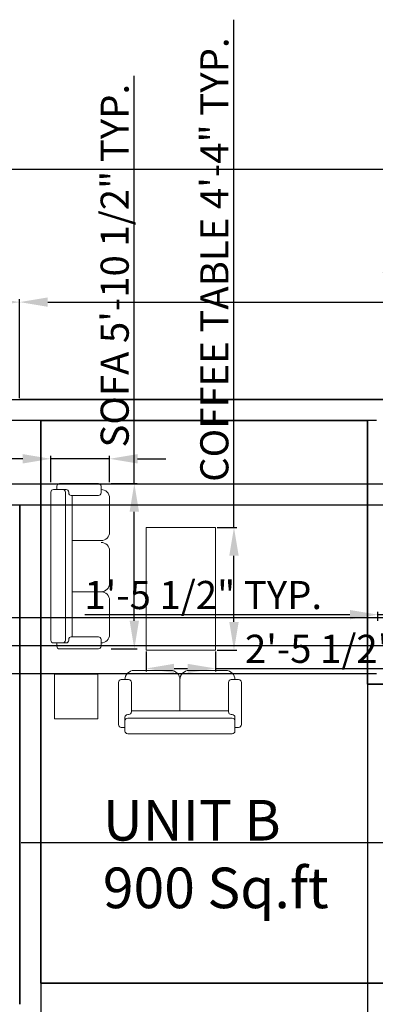
# Model space of a CAD drawing. Units: inches. Extents: x 2174 to 3353, y 1481 to 2316.
# Tile 7 of 8: x 2759 to 2911, y 1896 to 2316. Entities that reach past the tile are written whole.
import ezdxf

# ---------------------------------------------------------------- set-up
doc = ezdxf.new("R2010")
doc.units = ezdxf.units.IN
for name, color, linetype, lineweight in [('A-ANNO-DIMS', 2, 'Continuous', 18), ('A-AREA-IDEN', 7, 'Continuous', 25), ('A-FURN', 8, 'Continuous', 13), ('A-WALL', 7, 'Continuous', 35)]:
    doc.layers.add(name, color=color, linetype=linetype, lineweight=lineweight)
doc.styles.get("Standard").update_dxf_attribs({"font": 'arial.ttf'})
doc.dimstyles.new('ISO-25', dxfattribs={"dimtxt": 12, "dimasz": 12, "dimexe": 1.25, "dimexo": 0.625, "dimtad": 1, "dimlunit": 3, "dimtxsty": 'Standard', "dimcen": 2.5, "dimadec": 0, "dimazin": 0, "dimtfac": 1, "dimtmove": 0, "dimatfit": 3, "dimfxl": 1, "dimarcsym": 0})

# ---------------------------------------------------------------- blocks, each defined once
blk = doc.blocks.new('A$C115861F8')
for p, q in [((0, 0.572), (0, 0.126)), ((0.068, 0.601), (0.029, 0.601)), ((0.068, 0.64), (0.068, 0.601)), ((0.068, 0.533), (0.068, 0.601)), ((1.785, 0.669), (0.097, 0.669)), ((1.814, 0.64), (1.814, 0.601)), ((1.814, 0.601), (1.852, 0.601)), ((1.814, 0.533), (1.814, 0.601)), ((1.882, 0.572), (1.882, 0.126)), ((0.068, 0.495), (0.068, 0.543)), ((1.785, 0.504), (0.097, 0.504)), ((0.107, 0.466), (0.097, 0.466)), ((1.775, 0.466), (1.785, 0.466)), ((1.814, 0.495), (1.814, 0.543)), ((0.136, 0.126), (0.136, 0.436)), ((1.746, 0.427), (0.136, 0.427)), ((0.65, 0.097), (0.65, 0.427)), ((1.232, 0.097), (1.232, 0.427)), ((1.746, 0.126), (1.746, 0.436)), ((0.029, 0.097), (0.107, 0.097)), ((0.165, 0), (0.553, 0)), ((1.135, 0), (0.747, 0)), ((1.329, 0), (1.717, 0)), ((1.852, 0.097), (1.775, 0.097))]:
    blk.add_line(p, q)
for centre, radius, start, end in [((0.029, 0.572), 0.0291, 90, 180), ((0.097, 0.64), 0.0291, 90, 180), ((1.785, 0.64), 0.0291, 0, 90), ((1.852, 0.572), 0.0291, 0, 90), ((0.097, 0.533), 0.0291, 180, 270), ((0.097, 0.495), 0.0291, 180, 270), ((0.107, 0.436), 0.0291, 0, 90), ((1.775, 0.436), 0.0291, 90, 180), ((1.785, 0.533), 0.0291, 270, 0), ((1.785, 0.495), 0.0291, 270, 0), ((0.029, 0.126), 0.0291, 180, 270), ((0.107, 0.126), 0.0291, 270, 0), ((1.775, 0.126), 0.0291, 180, 270), ((1.852, 0.126), 0.0291, 270, 0), ((0.165, 0.097), 0.097, 180, 270), ((0.553, 0.097), 0.097, 270, 0), ((0.747, 0.097), 0.097, 180, 270), ((1.115, 0.097), 0.097, 270, 0), ((1.329, 0.097), 0.097, 180, 270), ((1.717, 0.097), 0.097, 270, 0)]:
    blk.add_arc(centre, radius, start, end)
blk = doc.blocks.new('A$C02A636C4')
for p, q in [((0.068, 0.64), (0.068, 0.601)), ((1.203, 0.669), (0.097, 0.669)), ((1.232, 0.64), (1.232, 0.601)), ((0, 0.572), (0, 0.126)), ((0.068, 0.601), (0.029, 0.601)), ((0.068, 0.533), (0.068, 0.601)), ((0.068, 0.495), (0.068, 0.543)), ((1.232, 0.601), (1.271, 0.601)), ((1.232, 0.533), (1.232, 0.601)), ((1.232, 0.495), (1.232, 0.543)), ((1.3, 0.572), (1.3, 0.126)), ((1.203, 0.504), (0.097, 0.504)), ((0.107, 0.466), (0.097, 0.466)), ((0.136, 0.126), (0.136, 0.436)), ((1.164, 0.427), (0.136, 0.427)), ((0.65, 0.097), (0.65, 0.427)), ((1.164, 0.126), (1.164, 0.436)), ((1.193, 0.466), (1.203, 0.466)), ((0.029, 0.097), (0.107, 0.097)), ((0.165, 0), (0.553, 0)), ((0.747, 0), (1.135, 0)), ((1.271, 0.097), (1.193, 0.097))]:
    blk.add_line(p, q)
for centre, radius, start, end in [((0.097, 0.64), 0.0291, 90, 180), ((1.203, 0.64), 0.0291, 0, 90), ((0.029, 0.572), 0.0291, 90, 180), ((0.097, 0.533), 0.0291, 180, 270), ((1.203, 0.533), 0.0291, 270, 0), ((1.271, 0.572), 0.0291, 0, 90), ((0.097, 0.495), 0.0291, 180, 270), ((0.107, 0.436), 0.0291, 0, 90), ((1.193, 0.436), 0.0291, 90, 180), ((1.203, 0.495), 0.0291, 270, 0), ((0.029, 0.126), 0.0291, 180, 270), ((0.107, 0.126), 0.0291, 270, 0), ((1.193, 0.126), 0.0291, 180, 270), ((1.271, 0.126), 0.0291, 270, 0), ((0.165, 0.097), 0.097, 180, 270), ((0.553, 0.097), 0.097, 270, 0), ((0.747, 0.097), 0.097, 180, 270), ((1.135, 0.097), 0.097, 270, 0)]:
    blk.add_arc(centre, radius, start, end)
blk = doc.blocks.new('*D7')
at = {"layer": 'A-ANNO-DIMS', "color": 0, "lineweight": -2, "transparency": 16777216}
for p, q in [((2285.44, 2154.23), (2285.44, 2253.16)), ((2297.44, 2251.91), (3092.44, 2251.91)), ((3104.44, 2154.23), (3104.44, 2253.16))]:
    blk.add_line(p, q, dxfattribs=at)
at = {"layer": 'A-ANNO-DIMS', "color": 0, "transparency": 16777216}
for points in [[(2297.44, 2253.91), (2297.44, 2249.91), (2285.44, 2251.91)], [(3092.44, 2253.91), (3092.44, 2249.91), (3104.44, 2251.91)]]:
    blk.add_solid(points, dxfattribs=at)
at = {"layer": 'Defpoints', "color": 0, "transparency": 16777216}
for p in [(3104.44, 2251.91), (2285.44, 2153.61), (3104.44, 2153.61)]:
    blk.add_point(p, dxfattribs=at)
at = {"layer": 'A-ANNO-DIMS', "color": 0, "transparency": 16777216, "insert": (2694.94, 2258.66), "char_height": 12, "attachment_point": 5}
blk.add_mtext('68\'-3"', dxfattribs=at)
blk = doc.blocks.new('TABLE-COFFEE')
blk.add_lwpolyline([(0, 52.25), (29.71, 52.25), (29.71, 0), (0, 0)], close=True)
blk = doc.blocks.new('*D15')
at = {"layer": 'A-ANNO-DIMS', "color": 0, "lineweight": -2, "transparency": 16777216}
for p, q in [((2933.04, 2070.53), (2933.04, 2209.98)), ((2930.38, 2058.53), (2934.29, 2058.53)), ((2933.04, 2036.61), (2933.04, 2058.53)), ((2930.38, 2036.61), (2934.29, 2036.61)), ((2933.04, 2024.61), (2933.04, 2012.61))]:
    blk.add_line(p, q, dxfattribs=at)
at = {"layer": 'A-ANNO-DIMS', "color": 0, "transparency": 16777216}
for points in [[(2931.04, 2070.53), (2935.04, 2070.53), (2933.04, 2058.53)], [(2931.04, 2024.61), (2935.04, 2024.61), (2933.04, 2036.61)]]:
    blk.add_solid(points, dxfattribs=at)
at = {"layer": 'Defpoints', "color": 0, "transparency": 16777216}
for p in [(2929.75, 2058.53), (2933.04, 2058.53), (2929.75, 2036.61)]:
    blk.add_point(p, dxfattribs=at)
at = {"layer": 'A-ANNO-DIMS', "color": 0, "transparency": 16777216, "insert": (2926.21, 2146.25), "char_height": 12, "attachment_point": 5, "rotation": 90}
blk.add_mtext('SINK 1\'-10" TYP.', dxfattribs=at)
blk = doc.blocks.new('*D16')
at = {"layer": 'A-ANNO-DIMS', "color": 0, "lineweight": -2, "transparency": 16777216}
for p, q in [((2912.44, 2059.16), (2912.44, 2063.07)), ((2929.75, 2059.16), (2929.75, 2063.07)), ((2900.44, 2061.82), (2787.22, 2061.82)), ((2929.75, 2061.82), (2912.44, 2061.82)), ((2941.75, 2061.82), (2953.75, 2061.82))]:
    blk.add_line(p, q, dxfattribs=at)
at = {"layer": 'A-ANNO-DIMS', "color": 0, "transparency": 16777216}
for points in [[(2900.44, 2063.82), (2900.44, 2059.82), (2912.44, 2061.82)], [(2941.75, 2063.82), (2941.75, 2059.82), (2929.75, 2061.82)]]:
    blk.add_solid(points, dxfattribs=at)
at = {"layer": 'Defpoints', "color": 0, "transparency": 16777216}
for p in [(2912.44, 2061.82), (2912.44, 2058.53), (2929.75, 2058.53)]:
    blk.add_point(p, dxfattribs=at)
at = {"layer": 'A-ANNO-DIMS', "color": 0, "transparency": 16777216, "insert": (2837.83, 2068.65), "char_height": 12, "attachment_point": 5}
blk.add_mtext('1\'-5 1/2" TYP.', dxfattribs=at)
blk = doc.blocks.new('*D19')
at = {"layer": 'A-ANNO-DIMS', "color": 0, "lineweight": -2, "transparency": 16777216}
for p, q in [((2808.4, 2117.73), (2808.4, 2291.66)), ((2798.45, 2117.73), (2809.65, 2117.73)), ((2808.4, 2059.24), (2808.4, 2105.73)), ((2798.45, 2047.24), (2809.65, 2047.24))]:
    blk.add_line(p, q, dxfattribs=at)
at = {"layer": 'A-ANNO-DIMS', "color": 0, "transparency": 16777216}
for points in [[(2806.4, 2105.73), (2810.4, 2105.73), (2808.4, 2117.73)], [(2806.4, 2059.24), (2810.4, 2059.24), (2808.4, 2047.24)]]:
    blk.add_solid(points, dxfattribs=at)
at = {"layer": 'Defpoints', "color": 0, "transparency": 16777216}
for p in [(2797.83, 2117.73), (2808.4, 2117.73), (2797.83, 2047.24)]:
    blk.add_point(p, dxfattribs=at)
at = {"layer": 'A-ANNO-DIMS', "color": 0, "transparency": 16777216, "insert": (2801.57, 2210.69), "char_height": 12, "attachment_point": 5, "rotation": 90}
blk.add_mtext('SOFA 5\'-10 1/2" TYP.', dxfattribs=at)
blk = doc.blocks.new('*D20')
at = {"layer": 'A-ANNO-DIMS', "color": 0, "lineweight": -2, "transparency": 16777216}
for p, q in [((2772.76, 2118.36), (2772.76, 2129.56)), ((2797.83, 2118.36), (2797.83, 2129.56)), ((2760.76, 2128.31), (2674.16, 2128.31)), ((2797.83, 2128.31), (2772.76, 2128.31)), ((2809.83, 2128.31), (2821.83, 2128.31))]:
    blk.add_line(p, q, dxfattribs=at)
at = {"layer": 'A-ANNO-DIMS', "color": 0, "transparency": 16777216}
for points in [[(2760.76, 2130.31), (2760.76, 2126.31), (2772.76, 2128.31)], [(2809.83, 2130.31), (2809.83, 2126.31), (2797.83, 2128.31)]]:
    blk.add_solid(points, dxfattribs=at)
at = {"layer": 'Defpoints', "color": 0, "transparency": 16777216}
for p in [(2772.76, 2128.31), (2772.76, 2117.73), (2797.83, 2117.73)]:
    blk.add_point(p, dxfattribs=at)
at = {"layer": 'A-ANNO-DIMS', "color": 0, "transparency": 16777216, "insert": (2711.46, 2134.96), "char_height": 12, "attachment_point": 5}
blk.add_mtext('2\'-1" TYP.', dxfattribs=at)
blk = doc.blocks.new('*D33')
at = {"layer": 'A-ANNO-DIMS', "color": 0, "lineweight": -2, "transparency": 16777216}
for p, q in [((2850.96, 2098.96), (2850.96, 2315.63)), ((2843.75, 2098.96), (2852.21, 2098.96)), ((2850.96, 2058.71), (2850.96, 2086.96)), ((2843.75, 2046.71), (2852.21, 2046.71))]:
    blk.add_line(p, q, dxfattribs=at)
at = {"layer": 'A-ANNO-DIMS', "color": 0, "transparency": 16777216}
for points in [[(2848.96, 2086.96), (2852.96, 2086.96), (2850.96, 2098.96)], [(2848.96, 2058.71), (2852.96, 2058.71), (2850.96, 2046.71)]]:
    blk.add_solid(points, dxfattribs=at)
at = {"layer": 'Defpoints', "color": 0, "transparency": 16777216}
for p in [(2843.12, 2098.96), (2850.96, 2098.96), (2843.12, 2046.71)]:
    blk.add_point(p, dxfattribs=at)
at = {"layer": 'A-ANNO-DIMS', "color": 0, "transparency": 16777216, "insert": (2844.13, 2213.29), "char_height": 12, "attachment_point": 5, "rotation": 90}
blk.add_mtext('COFFEE TABLE 4\'-4" TYP.', dxfattribs=at)
blk = doc.blocks.new('*D34')
at = {"layer": 'A-ANNO-DIMS', "color": 0, "lineweight": -2, "transparency": 16777216}
for p, q in [((2813.41, 2046.08), (2813.41, 2037.62)), ((2843.12, 2046.08), (2843.12, 2037.62)), ((2825.41, 2038.87), (2831.12, 2038.87)), ((2843.12, 2038.87), (2957.69, 2038.87))]:
    blk.add_line(p, q, dxfattribs=at)
at = {"layer": 'A-ANNO-DIMS', "color": 0, "transparency": 16777216}
for points in [[(2825.41, 2040.87), (2825.41, 2036.87), (2813.41, 2038.87)], [(2831.12, 2040.87), (2831.12, 2036.87), (2843.12, 2038.87)]]:
    blk.add_solid(points, dxfattribs=at)
at = {"layer": 'Defpoints', "color": 0, "transparency": 16777216}
for p in [(2813.41, 2046.71), (2843.12, 2046.71), (2843.12, 2038.87)]:
    blk.add_point(p, dxfattribs=at)
at = {"layer": 'A-ANNO-DIMS', "color": 0, "transparency": 16777216, "insert": (2906.41, 2045.7), "char_height": 12, "attachment_point": 5}
blk.add_mtext('2\'-5 1/2" TYP.', dxfattribs=at)
blk = doc.blocks.new('*D45')
at = {"layer": 'A-ANNO-DIMS', "color": 0, "lineweight": -2, "transparency": 16777216}
for p, q in [((2639.44, 2154.23), (2639.44, 2196.41)), ((2651.44, 2195.16), (2747.44, 2195.16)), ((2759.44, 2154.23), (2759.44, 2196.41))]:
    blk.add_line(p, q, dxfattribs=at)
at = {"layer": 'A-ANNO-DIMS', "color": 0, "transparency": 16777216}
for points in [[(2651.44, 2197.16), (2651.44, 2193.16), (2639.44, 2195.16)], [(2747.44, 2197.16), (2747.44, 2193.16), (2759.44, 2195.16)]]:
    blk.add_solid(points, dxfattribs=at)
at = {"layer": 'Defpoints', "color": 0, "transparency": 16777216}
for p in [(2759.44, 2195.16), (2639.44, 2153.61), (2759.44, 2153.61)]:
    blk.add_point(p, dxfattribs=at)
at = {"layer": 'A-ANNO-DIMS', "color": 0, "transparency": 16777216, "insert": (2699.44, 2201.91), "char_height": 12, "attachment_point": 5}
blk.add_mtext('10\'-0"', dxfattribs=at)
blk = doc.blocks.new('*D46')
at = {"layer": 'A-ANNO-DIMS', "color": 0, "lineweight": -2, "transparency": 16777216}
for p, q in [((2759.44, 2154.23), (2759.44, 2196.41)), ((2771.44, 2195.16), (3101.44, 2195.16)), ((3113.44, 2154.23), (3113.44, 2196.41))]:
    blk.add_line(p, q, dxfattribs=at)
at = {"layer": 'A-ANNO-DIMS', "color": 0, "transparency": 16777216}
for points in [[(2771.44, 2197.16), (2771.44, 2193.16), (2759.44, 2195.16)], [(3101.44, 2197.16), (3101.44, 2193.16), (3113.44, 2195.16)]]:
    blk.add_solid(points, dxfattribs=at)
at = {"layer": 'Defpoints', "color": 0, "transparency": 16777216}
for p in [(3113.44, 2195.16), (2759.44, 2153.61), (3113.44, 2153.61)]:
    blk.add_point(p, dxfattribs=at)
at = {"layer": 'A-ANNO-DIMS', "color": 0, "transparency": 16777216, "insert": (2936.44, 2201.91), "char_height": 12, "attachment_point": 5}
blk.add_mtext('29\'-6"', dxfattribs=at)
blk = doc.blocks.new('*D47')
at = {"layer": 'A-ANNO-DIMS', "color": 0, "lineweight": -2, "transparency": 16777216}
for p, q in [((2640.07, 2153.61), (3156.24, 2153.61)), ((3154.99, 2141.61), (3154.99, 2129.61)), ((2640.07, 2117.61), (3156.24, 2117.61))]:
    blk.add_line(p, q, dxfattribs=at)
at = {"layer": 'A-ANNO-DIMS', "color": 0, "transparency": 16777216}
for points in [[(3152.99, 2141.61), (3156.99, 2141.61), (3154.99, 2153.61)], [(3152.99, 2129.61), (3156.99, 2129.61), (3154.99, 2117.61)]]:
    blk.add_solid(points, dxfattribs=at)
at = {"layer": 'Defpoints', "color": 0, "transparency": 16777216}
for p in [(2639.44, 2153.61), (2639.44, 2117.61), (3154.99, 2117.61)]:
    blk.add_point(p, dxfattribs=at)
at = {"layer": 'A-ANNO-DIMS', "color": 0, "transparency": 16777216, "insert": (3148.24, 2135.61), "char_height": 12, "attachment_point": 5, "rotation": 90}
blk.add_mtext('3\'-0"', dxfattribs=at)
blk = doc.blocks.new('*D55')
at = {"layer": 'A-ANNO-DIMS', "color": 0, "lineweight": -2, "transparency": 16777216}
for p, q in [((2768.44, 2143.98), (2768.44, 1510.81)), ((2907.94, 2143.98), (2907.94, 1510.81)), ((2780.44, 1512.06), (2895.94, 1512.06))]:
    blk.add_line(p, q, dxfattribs=at)
at = {"layer": 'A-ANNO-DIMS', "color": 0, "transparency": 16777216}
for points in [[(2780.44, 1514.06), (2780.44, 1510.06), (2768.44, 1512.06)], [(2895.94, 1514.06), (2895.94, 1510.06), (2907.94, 1512.06)]]:
    blk.add_solid(points, dxfattribs=at)
at = {"layer": 'Defpoints', "color": 0, "transparency": 16777216}
for p in [(2768.44, 2144.61), (2907.94, 2144.61), (2907.94, 1512.06)]:
    blk.add_point(p, dxfattribs=at)
at = {"layer": 'A-ANNO-DIMS', "color": 0, "transparency": 16777216, "insert": (2838.19, 1518.89), "char_height": 12, "attachment_point": 5}
blk.add_mtext('11\'-7 1/2"', dxfattribs=at)
blk = doc.blocks.new('*D59')
at = {"layer": 'A-ANNO-DIMS', "color": 0, "lineweight": -2, "transparency": 16777216}
for p, q in [((2911.82, 2144.61), (2242.64, 2144.61)), ((2243.89, 2048.61), (2243.89, 2132.61)), ((2911.82, 2036.61), (2242.64, 2036.61))]:
    blk.add_line(p, q, dxfattribs=at)
at = {"layer": 'A-ANNO-DIMS', "color": 0, "transparency": 16777216}
for points in [[(2241.89, 2132.61), (2245.89, 2132.61), (2243.89, 2144.61)], [(2241.89, 2048.61), (2245.89, 2048.61), (2243.89, 2036.61)]]:
    blk.add_solid(points, dxfattribs=at)
at = {"layer": 'Defpoints', "color": 0, "transparency": 16777216}
for p in [(2243.89, 2144.61), (2912.44, 2144.61), (2912.44, 2036.61)]:
    blk.add_point(p, dxfattribs=at)
at = {"layer": 'A-ANNO-DIMS', "color": 0, "transparency": 16777216, "insert": (2237.14, 2090.61), "char_height": 12, "attachment_point": 5, "rotation": 90}
blk.add_mtext('9\'-0"', dxfattribs=at)
blk = doc.blocks.new('*D69')
at = {"layer": 'A-ANNO-DIMS', "color": 0, "lineweight": -2, "transparency": 16777216}
for p, q in [((2640.07, 2108.61), (3156.24, 2108.61)), ((3154.99, 2072.61), (3154.99, 2096.61)), ((2640.07, 2060.61), (3156.24, 2060.61))]:
    blk.add_line(p, q, dxfattribs=at)
at = {"layer": 'A-ANNO-DIMS', "color": 0, "transparency": 16777216}
for points in [[(3152.99, 2096.61), (3156.99, 2096.61), (3154.99, 2108.61)], [(3152.99, 2072.61), (3156.99, 2072.61), (3154.99, 2060.61)]]:
    blk.add_solid(points, dxfattribs=at)
at = {"layer": 'Defpoints', "color": 0, "transparency": 16777216}
for p in [(2639.44, 2108.61), (3154.99, 2108.61), (2639.44, 2060.61)]:
    blk.add_point(p, dxfattribs=at)
at = {"layer": 'A-ANNO-DIMS', "color": 0, "transparency": 16777216, "insert": (3148.24, 2084.61), "char_height": 12, "attachment_point": 5, "rotation": 90}
blk.add_mtext('4\'-0"', dxfattribs=at)
blk = doc.blocks.new('*D70')
at = {"layer": 'A-ANNO-DIMS', "color": 0, "lineweight": -2, "transparency": 16777216}
for p, q in [((2760.07, 2060.61), (3156.24, 2060.61)), ((3154.99, 1976.61), (3154.99, 2048.61)), ((2760.07, 1964.61), (3156.24, 1964.61))]:
    blk.add_line(p, q, dxfattribs=at)
at = {"layer": 'A-ANNO-DIMS', "color": 0, "transparency": 16777216}
for points in [[(3152.99, 2048.61), (3156.99, 2048.61), (3154.99, 2060.61)], [(3152.99, 1976.61), (3156.99, 1976.61), (3154.99, 1964.61)]]:
    blk.add_solid(points, dxfattribs=at)
at = {"layer": 'Defpoints', "color": 0, "transparency": 16777216}
for p in [(2759.44, 2060.61), (3154.99, 2060.61), (2759.44, 1964.61)]:
    blk.add_point(p, dxfattribs=at)
at = {"layer": 'A-ANNO-DIMS', "color": 0, "transparency": 16777216, "insert": (3148.24, 2012.61), "char_height": 12, "attachment_point": 5, "rotation": 90}
blk.add_mtext('8\'-0"', dxfattribs=at)
blk = doc.blocks.new('*D71')
at = {"layer": 'A-ANNO-DIMS', "color": 0, "lineweight": -2, "transparency": 16777216}
for p, q in [((3154.99, 2072.61), (3154.99, 2084.61)), ((2640.07, 2060.61), (3156.24, 2060.61)), ((3154.99, 2060.61), (3154.99, 2048.61)), ((2640.07, 2048.61), (3156.24, 2048.61)), ((3154.99, 2036.61), (3154.99, 1992.59))]:
    blk.add_line(p, q, dxfattribs=at)
at = {"layer": 'A-ANNO-DIMS', "color": 0, "transparency": 16777216}
for points in [[(3152.99, 2072.61), (3156.99, 2072.61), (3154.99, 2060.61)], [(3152.99, 2036.61), (3156.99, 2036.61), (3154.99, 2048.61)]]:
    blk.add_solid(points, dxfattribs=at)
at = {"layer": 'Defpoints', "color": 0, "transparency": 16777216}
for p in [(2639.44, 2060.61), (2639.44, 2048.61), (3154.99, 2048.61)]:
    blk.add_point(p, dxfattribs=at)
at = {"layer": 'A-ANNO-DIMS', "color": 0, "transparency": 16777216, "insert": (3148.24, 2008.6), "char_height": 12, "attachment_point": 5, "rotation": 90}
blk.add_mtext('1\'-0"', dxfattribs=at)

msp = doc.modelspace()

# ---------------------------------------------------------------- linework, layer by layer
at = {"layer": 'A-FURN'}
msp.add_lwpolyline([(2774.296, 2036.392), (2792.77, 2036.392), (2792.77, 2017.374), (2774.296, 2017.374)], close=True, dxfattribs=at)
at = {"layer": 'A-WALL'}
for p, q in [((2759.444, 2153.608), (3113.444, 2153.608)), ((2768.444, 2144.608), (2768.444, 1904.608)), ((2768.444, 2144.608), (2907.944, 2144.608)), ((2907.944, 2144.608), (2907.944, 2032.108)), ((2759.444, 2108.608), (2759.444, 1895.608)), ((2907.944, 2032.108), (2936.444, 2032.108)), ((2768.444, 1904.608), (3008.444, 1904.608))]:
    msp.add_line(p, q, dxfattribs=at)

# ---------------------------------------------------------------- block references
at = {"layer": 'A-FURN'}
for name, p, xscale, yscale, zscale, rotation in [('A$C115861F8', (2797.829, 2047.236), 37.46691384636836, 37.46691384636836, 37.46691384636836, 89.99999999999999), ('A$C02A636C4', (2854.126, 2038.016), 40.36195249324395, 40.36195249324395, 40.36195249324395, 180)]:
    msp.add_blockref(name, p, dxfattribs=dict(at, xscale=xscale, yscale=yscale, zscale=zscale, rotation=rotation))
msp.add_blockref('TABLE-COFFEE', (2813.413, 2046.708), dxfattribs=at)

# ---------------------------------------------------------------- texts
at = {"layer": 'A-AREA-IDEN', "insert": (2794.974, 1982.768), "char_height": 17.3039, "attachment_point": 1}
msp.add_mtext_dynamic_manual_height_columns('UNIT B \\P900 Sq.ft', width=375.7284, gutter_width=86.519, heights=[0], dxfattribs=at)

# ---------------------------------------------------------------- dimensions: what is measured, and where the dimension line sits
at = {"layer": 'A-ANNO-DIMS'}
for base, p1, p2, angle, text, picture, middle in [((2850.9623, 2098.9576), (2843.1248, 2046.7077), (2843.1248, 2098.9576), 90, 'COFFEE TABLE <> TYP.', '*D33', (2844.1285, 2213.292)), ((2808.404, 2117.732), (2797.829, 2047.236), (2797.829, 2117.732), 90, 'SOFA <> TYP.', '*D19', (2801.57, 2210.694)), ((2933.041, 2058.531), (2929.752, 2036.608), (2929.752, 2058.531), 90, 'SINK <> TYP.', '*D15', (2926.211, 2146.254)), ((2772.756, 2128.306), (2797.829, 2117.732), (2772.756, 2117.732), 180, '<> TYP.', '*D20', (2711.456, 2134.96)), ((2912.444, 2061.82), (2929.752, 2058.531), (2912.444, 2058.531), 180, '<> TYP.', '*D16', (2837.83, 2068.649))]:
    dim = msp.add_linear_dim(base=base, p1=p1, p2=p2, angle=angle, text=text, dimstyle='ISO-25', override={"dimdec": 1, "dimlfac": 1, "dimrnd": 0, "dimzin": 1, "dimdsep": 46, "dimlunit": 4, "dimfrac": 2}, dxfattribs=at)
    dim.commit()
    dim.dimension.update_dxf_attribs({"geometry": picture, "text_midpoint": middle})
for base, p1, p2, override, picture, middle in [((3104.444, 2251.907), (2285.444, 2153.608), (3104.444, 2153.608), {"dimclrd": 0, "dimclre": 0, "dimclrt": 0}, '*D7', (2694.944, 2258.663)), ((2759.444, 2195.158), (2639.444, 2153.608), (2759.444, 2153.608), {"dimdec": 1, "dimlfac": 1, "dimrnd": 0, "dimzin": 1, "dimdsep": 46, "dimlunit": 4, "dimfrac": 2}, '*D45', (2699.444, 2201.909)), ((3113.444, 2195.158), (2759.444, 2153.608), (3113.444, 2153.608), {"dimdec": 1, "dimlfac": 1, "dimrnd": 0, "dimzin": 1, "dimdsep": 46, "dimlunit": 4, "dimfrac": 2}, '*D46', (2936.444, 2201.909)), ((2907.944, 1512.058), (2768.444, 2144.608), (2907.944, 2144.608), {"dimdec": 1, "dimlfac": 1, "dimrnd": 0, "dimzin": 1, "dimdsep": 46, "dimlunit": 4, "dimfrac": 2}, '*D55', (2838.194, 1518.887))]:
    dim = msp.add_linear_dim(base=base, p1=p1, p2=p2, dimstyle='ISO-25', override=override, dxfattribs=at)
    dim.commit()
    dim.dimension.update_dxf_attribs({"geometry": picture, "text_midpoint": middle})
for base, p1, p2, picture, middle in [((3154.994, 2117.608), (2639.444, 2153.608), (2639.444, 2117.608), '*D47', (3148.238, 2135.608)), ((2243.894, 2144.608), (2912.444, 2036.608), (2912.444, 2144.608), '*D59', (2237.143, 2090.608)), ((3154.994, 2108.608), (2639.444, 2060.608), (2639.444, 2108.608), '*D69', (3148.243, 2084.608)), ((3154.994, 2048.608), (2639.444, 2060.608), (2639.444, 2048.608), '*D71', (3148.243, 2008.598)), ((3154.994, 2060.608), (2759.444, 1964.608), (2759.444, 2060.608), '*D70', (3148.243, 2012.608))]:
    dim = msp.add_linear_dim(base=base, p1=p1, p2=p2, angle=90, dimstyle='ISO-25', override={"dimdec": 1, "dimlfac": 1, "dimrnd": 0, "dimzin": 1, "dimdsep": 46, "dimlunit": 4, "dimfrac": 2}, dxfattribs=at)
    dim.commit()
    dim.dimension.update_dxf_attribs({"geometry": picture, "text_midpoint": middle})
dim = msp.add_linear_dim(base=(2843.125, 2038.87), p1=(2813.413, 2046.708), p2=(2843.125, 2046.708), text='<> TYP.', dimstyle='ISO-25', override={"dimdec": 1, "dimlfac": 1, "dimrnd": 0, "dimzin": 1, "dimdsep": 46, "dimlunit": 4, "dimfrac": 2}, dxfattribs=at)
dim.commit()
dim.dimension.update_dxf_attribs({"geometry": '*D34', "text_midpoint": (2906.406, 2045.7)})

doc.saveas('drawing.dxf')
